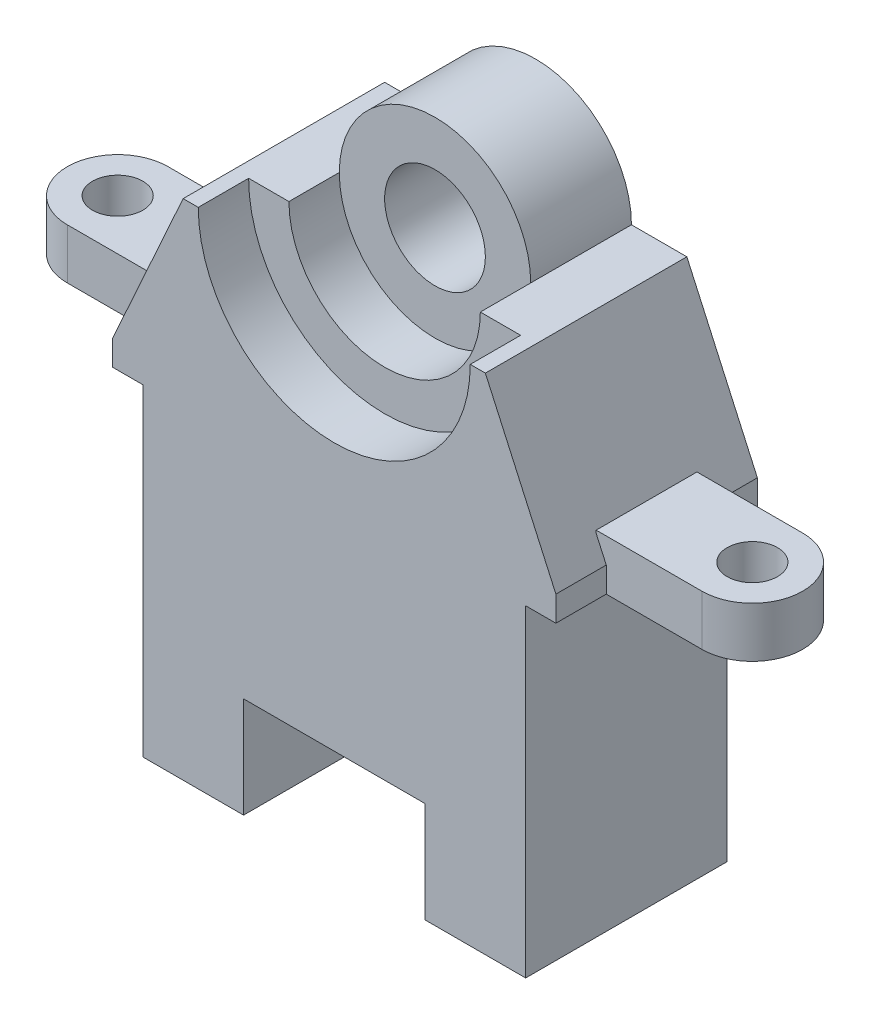
ISO-10303-21;
HEADER;
FILE_DESCRIPTION(('STEP AP214'),'2;1');
FILE_NAME('part.step','',(''),(''),'','','');
FILE_SCHEMA(('AUTOMOTIVE_DESIGN { 1 0 10303 214 1 1 1 1 }'));
ENDSEC;
DATA;
#1=APPLICATION_CONTEXT('core data for automotive mechanical design processes');
#2=APPLICATION_PROTOCOL_DEFINITION('international standard','automotive_design',2000,#1);
#3=PRODUCT_CONTEXT('',#1,'mechanical');
#4=PRODUCT('Part','Part','',(#3));
#5=PRODUCT_RELATED_PRODUCT_CATEGORY('part','',(#4));
#6=PRODUCT_DEFINITION_FORMATION('','',#4);
#7=PRODUCT_DEFINITION_CONTEXT('part definition',#1,'design');
#8=PRODUCT_DEFINITION('design','',#6,#7);
#9=PRODUCT_DEFINITION_SHAPE('','',#8);
#10=(LENGTH_UNIT() NAMED_UNIT(*) SI_UNIT(.MILLI.,.METRE.));
#11=(NAMED_UNIT(*) PLANE_ANGLE_UNIT() SI_UNIT($,.RADIAN.));
#12=(NAMED_UNIT(*) SI_UNIT($,.STERADIAN.) SOLID_ANGLE_UNIT());
#13=UNCERTAINTY_MEASURE_WITH_UNIT(LENGTH_MEASURE(1.E-05),#10,'distance_accuracy_value','');
#14=(GEOMETRIC_REPRESENTATION_CONTEXT(3) GLOBAL_UNCERTAINTY_ASSIGNED_CONTEXT((#13)) GLOBAL_UNIT_ASSIGNED_CONTEXT((#10,
#11,#12)) REPRESENTATION_CONTEXT('',''));
#15=CARTESIAN_POINT('',(0.,0.,0.));
#16=DIRECTION('',(0.,0.,1.));
#17=DIRECTION('',(1.,0.,0.));
#18=AXIS2_PLACEMENT_3D('',#15,#16,#17);
#19=CARTESIAN_POINT('',(38.,100.,0.));
#20=DIRECTION('',(0.,0.,1.));
#21=DIRECTION('',(1.,0.,0.));
#22=AXIS2_PLACEMENT_3D('',#19,#20,#21);
#23=CYLINDRICAL_SURFACE('',#22,19.);
#24=DIRECTION('',(0.,0.,1.));
#25=VECTOR('',#24,1.);
#26=CARTESIAN_POINT('',(19.,100.,0.));
#27=LINE('',#26,#25);
#28=CARTESIAN_POINT('',(19.,100.,0.));
#29=VERTEX_POINT('',#28);
#30=CARTESIAN_POINT('',(19.,100.,20.));
#31=VERTEX_POINT('',#30);
#32=EDGE_CURVE('E277',#29,#31,#27,.T.);
#33=ORIENTED_EDGE('',*,*,#32,.T.);
#34=CARTESIAN_POINT('',(38.,100.,20.));
#35=DIRECTION('',(0.,0.,1.));
#36=DIRECTION('',(1.,0.,0.));
#37=AXIS2_PLACEMENT_3D('',#34,#35,#36);
#38=CIRCLE('',#37,19.);
#39=CARTESIAN_POINT('',(57.,100.,20.));
#40=VERTEX_POINT('',#39);
#41=EDGE_CURVE('E1027',#40,#31,#38,.T.);
#42=ORIENTED_EDGE('',*,*,#41,.F.);
#43=DIRECTION('',(0.,0.,1.));
#44=VECTOR('',#43,1.);
#45=CARTESIAN_POINT('',(57.,100.,0.));
#46=LINE('',#45,#44);
#47=CARTESIAN_POINT('',(57.,100.,0.));
#48=VERTEX_POINT('',#47);
#49=EDGE_CURVE('E264',#48,#40,#46,.T.);
#50=ORIENTED_EDGE('',*,*,#49,.F.);
#51=CARTESIAN_POINT('',(38.,100.,0.));
#52=DIRECTION('',(0.,0.,1.));
#53=DIRECTION('',(1.,0.,0.));
#54=AXIS2_PLACEMENT_3D('',#51,#52,#53);
#55=CIRCLE('',#54,19.);
#56=EDGE_CURVE('E262',#48,#29,#55,.T.);
#57=ORIENTED_EDGE('',*,*,#56,.T.);
#58=EDGE_LOOP('',(#33,#42,#50,#57));
#59=FACE_BOUND('',#58,.T.);
#60=ADVANCED_FACE('F44',(#59),#23,.T.);
#61=CARTESIAN_POINT('',(38.,100.,0.));
#62=DIRECTION('',(0.,1.,0.));
#63=DIRECTION('',(0.,0.,1.));
#64=AXIS2_PLACEMENT_3D('',#61,#62,#63);
#65=PLANE('',#64);
#66=ORIENTED_EDGE('',*,*,#32,.F.);
#67=DIRECTION('',(-1.,0.,0.));
#68=VECTOR('',#67,1.);
#69=CARTESIAN_POINT('',(38.,100.,0.));
#70=LINE('',#69,#68);
#71=CARTESIAN_POINT('',(8.,100.,0.));
#72=VERTEX_POINT('',#71);
#73=EDGE_CURVE('E385',#29,#72,#70,.T.);
#74=ORIENTED_EDGE('',*,*,#73,.T.);
#75=DIRECTION('',(0.,0.,1.));
#76=VECTOR('',#75,1.);
#77=CARTESIAN_POINT('',(8.,100.,0.));
#78=LINE('',#77,#76);
#79=CARTESIAN_POINT('',(8.,100.,40.));
#80=VERTEX_POINT('',#79);
#81=EDGE_CURVE('E418',#72,#80,#78,.T.);
#82=ORIENTED_EDGE('',*,*,#81,.T.);
#83=DIRECTION('',(-1.,0.,0.));
#84=VECTOR('',#83,1.);
#85=CARTESIAN_POINT('',(38.,100.,40.));
#86=LINE('',#85,#84);
#87=CARTESIAN_POINT('',(11.,100.,40.));
#88=VERTEX_POINT('',#87);
#89=EDGE_CURVE('E397',#88,#80,#86,.T.);
#90=ORIENTED_EDGE('',*,*,#89,.F.);
#91=DIRECTION('',(0.,0.,1.));
#92=VECTOR('',#91,1.);
#93=CARTESIAN_POINT('',(11.,100.,30.));
#94=LINE('',#93,#92);
#95=CARTESIAN_POINT('',(11.,100.,30.));
#96=VERTEX_POINT('',#95);
#97=EDGE_CURVE('E272',#96,#88,#94,.T.);
#98=ORIENTED_EDGE('',*,*,#97,.F.);
#99=DIRECTION('',(-1.,0.,0.));
#100=VECTOR('',#99,1.);
#101=CARTESIAN_POINT('',(11.,100.,30.));
#102=LINE('',#101,#100);
#103=CARTESIAN_POINT('',(19.,100.,30.));
#104=VERTEX_POINT('',#103);
#105=EDGE_CURVE('E268',#104,#96,#102,.T.);
#106=ORIENTED_EDGE('',*,*,#105,.F.);
#107=EDGE_CURVE('E254',#31,#104,#27,.T.);
#108=ORIENTED_EDGE('',*,*,#107,.F.);
#109=EDGE_LOOP('',(#66,#74,#82,#90,#98,#106,#108));
#110=FACE_BOUND('',#109,.T.);
#111=ADVANCED_FACE('F531',(#110),#65,.T.);
#112=CARTESIAN_POINT('',(82.,64.,0.));
#113=DIRECTION('',(1.,0.,0.));
#114=DIRECTION('',(0.,0.,-1.));
#115=AXIS2_PLACEMENT_3D('',#112,#113,#114);
#116=PLANE('',#115);
#117=DIRECTION('',(0.,-1.,0.));
#118=VECTOR('',#117,1.);
#119=CARTESIAN_POINT('',(82.,69.,30.));
#120=LINE('',#119,#118);
#121=CARTESIAN_POINT('',(82.,69.,30.));
#122=VERTEX_POINT('',#121);
#123=CARTESIAN_POINT('',(82.,64.,30.));
#124=VERTEX_POINT('',#123);
#125=EDGE_CURVE('E315',#122,#124,#120,.T.);
#126=ORIENTED_EDGE('',*,*,#125,.F.);
#127=DIRECTION('',(0.,0.,1.));
#128=VECTOR('',#127,1.);
#129=CARTESIAN_POINT('',(82.,69.,0.));
#130=LINE('',#129,#128);
#131=CARTESIAN_POINT('',(82.,69.,40.));
#132=VERTEX_POINT('',#131);
#133=EDGE_CURVE('E426',#122,#132,#130,.T.);
#134=ORIENTED_EDGE('',*,*,#133,.T.);
#135=DIRECTION('',(0.,1.,0.));
#136=VECTOR('',#135,1.);
#137=CARTESIAN_POINT('',(82.,64.,40.));
#138=LINE('',#137,#136);
#139=CARTESIAN_POINT('',(82.,64.,40.));
#140=VERTEX_POINT('',#139);
#141=EDGE_CURVE('E371',#140,#132,#138,.T.);
#142=ORIENTED_EDGE('',*,*,#141,.F.);
#143=DIRECTION('',(0.,0.,1.));
#144=VECTOR('',#143,1.);
#145=CARTESIAN_POINT('',(82.,64.,0.));
#146=LINE('',#145,#144);
#147=EDGE_CURVE('E393',#124,#140,#146,.T.);
#148=ORIENTED_EDGE('',*,*,#147,.F.);
#149=EDGE_LOOP('',(#126,#134,#142,#148));
#150=FACE_BOUND('',#149,.T.);
#151=ADVANCED_FACE('F540',(#150),#116,.T.);
#152=CARTESIAN_POINT('',(-6.,64.,0.));
#153=DIRECTION('',(-1.,0.,0.));
#154=DIRECTION('',(0.,0.,1.));
#155=AXIS2_PLACEMENT_3D('',#152,#153,#154);
#156=PLANE('',#155);
#157=DIRECTION('',(0.,-1.,0.));
#158=VECTOR('',#157,1.);
#159=CARTESIAN_POINT('',(-6.,69.,10.));
#160=LINE('',#159,#158);
#161=CARTESIAN_POINT('',(-6.,69.,10.));
#162=VERTEX_POINT('',#161);
#163=CARTESIAN_POINT('',(-6.,64.,10.));
#164=VERTEX_POINT('',#163);
#165=EDGE_CURVE('E356',#162,#164,#160,.T.);
#166=ORIENTED_EDGE('',*,*,#165,.F.);
#167=DIRECTION('',(0.,0.,1.));
#168=VECTOR('',#167,1.);
#169=CARTESIAN_POINT('',(-6.,69.,0.));
#170=LINE('',#169,#168);
#171=CARTESIAN_POINT('',(-6.,69.,0.));
#172=VERTEX_POINT('',#171);
#173=EDGE_CURVE('E412',#172,#162,#170,.T.);
#174=ORIENTED_EDGE('',*,*,#173,.F.);
#175=DIRECTION('',(0.,-1.,0.));
#176=VECTOR('',#175,1.);
#177=CARTESIAN_POINT('',(-6.,64.,0.));
#178=LINE('',#177,#176);
#179=CARTESIAN_POINT('',(-6.,64.,0.));
#180=VERTEX_POINT('',#179);
#181=EDGE_CURVE('E389',#172,#180,#178,.T.);
#182=ORIENTED_EDGE('',*,*,#181,.T.);
#183=DIRECTION('',(0.,0.,1.));
#184=VECTOR('',#183,1.);
#185=CARTESIAN_POINT('',(-6.,64.,0.));
#186=LINE('',#185,#184);
#187=EDGE_CURVE('E413',#180,#164,#186,.T.);
#188=ORIENTED_EDGE('',*,*,#187,.T.);
#189=EDGE_LOOP('',(#166,#174,#182,#188));
#190=FACE_BOUND('',#189,.T.);
#191=ADVANCED_FACE('F499',(#190),#156,.T.);
#192=CARTESIAN_POINT('',(20.,0.,40.));
#193=DIRECTION('',(0.,1.,0.));
#194=DIRECTION('',(0.,0.,1.));
#195=AXIS2_PLACEMENT_3D('',#192,#193,#194);
#196=PLANE('',#195);
#197=DIRECTION('',(1.,0.,0.));
#198=VECTOR('',#197,1.);
#199=CARTESIAN_POINT('',(20.,0.,0.));
#200=LINE('',#199,#198);
#201=CARTESIAN_POINT('',(0.,0.,0.));
#202=VERTEX_POINT('',#201);
#203=CARTESIAN_POINT('',(20.,0.,0.));
#204=VERTEX_POINT('',#203);
#205=EDGE_CURVE('E411',#202,#204,#200,.T.);
#206=ORIENTED_EDGE('',*,*,#205,.T.);
#207=DIRECTION('',(0.,0.,-1.));
#208=VECTOR('',#207,1.);
#209=CARTESIAN_POINT('',(20.,0.,40.));
#210=LINE('',#209,#208);
#211=CARTESIAN_POINT('',(20.,0.,40.));
#212=VERTEX_POINT('',#211);
#213=EDGE_CURVE('E481',#212,#204,#210,.T.);
#214=ORIENTED_EDGE('',*,*,#213,.F.);
#215=DIRECTION('',(1.,0.,0.));
#216=VECTOR('',#215,1.);
#217=CARTESIAN_POINT('',(20.,0.,40.));
#218=LINE('',#217,#216);
#219=CARTESIAN_POINT('',(0.,0.,40.));
#220=VERTEX_POINT('',#219);
#221=EDGE_CURVE('E435',#220,#212,#218,.T.);
#222=ORIENTED_EDGE('',*,*,#221,.F.);
#223=DIRECTION('',(0.,0.,-1.));
#224=VECTOR('',#223,1.);
#225=CARTESIAN_POINT('',(0.,0.,40.));
#226=LINE('',#225,#224);
#227=EDGE_CURVE('E449',#220,#202,#226,.T.);
#228=ORIENTED_EDGE('',*,*,#227,.T.);
#229=EDGE_LOOP('',(#206,#214,#222,#228));
#230=FACE_BOUND('',#229,.T.);
#231=ADVANCED_FACE('F50',(#230),#196,.F.);
#232=CARTESIAN_POINT('',(20.,20.,40.));
#233=DIRECTION('',(-1.,0.,0.));
#234=DIRECTION('',(0.,0.,1.));
#235=AXIS2_PLACEMENT_3D('',#232,#233,#234);
#236=PLANE('',#235);
#237=DIRECTION('',(0.,1.,0.));
#238=VECTOR('',#237,1.);
#239=CARTESIAN_POINT('',(20.,20.,0.));
#240=LINE('',#239,#238);
#241=CARTESIAN_POINT('',(20.,20.,0.));
#242=VERTEX_POINT('',#241);
#243=EDGE_CURVE('E451',#204,#242,#240,.T.);
#244=ORIENTED_EDGE('',*,*,#243,.T.);
#245=DIRECTION('',(0.,0.,-1.));
#246=VECTOR('',#245,1.);
#247=CARTESIAN_POINT('',(20.,20.,40.));
#248=LINE('',#247,#246);
#249=CARTESIAN_POINT('',(20.,20.,40.));
#250=VERTEX_POINT('',#249);
#251=EDGE_CURVE('E476',#250,#242,#248,.T.);
#252=ORIENTED_EDGE('',*,*,#251,.F.);
#253=DIRECTION('',(0.,1.,0.));
#254=VECTOR('',#253,1.);
#255=CARTESIAN_POINT('',(20.,20.,40.));
#256=LINE('',#255,#254);
#257=EDGE_CURVE('E434',#212,#250,#256,.T.);
#258=ORIENTED_EDGE('',*,*,#257,.F.);
#259=ORIENTED_EDGE('',*,*,#213,.T.);
#260=EDGE_LOOP('',(#244,#252,#258,#259));
#261=FACE_BOUND('',#260,.T.);
#262=ADVANCED_FACE('F892',(#261),#236,.F.);
#263=CARTESIAN_POINT('',(56.,20.,40.));
#264=DIRECTION('',(0.,1.,0.));
#265=DIRECTION('',(0.,0.,1.));
#266=AXIS2_PLACEMENT_3D('',#263,#264,#265);
#267=PLANE('',#266);
#268=DIRECTION('',(1.,0.,0.));
#269=VECTOR('',#268,1.);
#270=CARTESIAN_POINT('',(56.,20.,0.));
#271=LINE('',#270,#269);
#272=CARTESIAN_POINT('',(56.,20.,0.));
#273=VERTEX_POINT('',#272);
#274=EDGE_CURVE('E454',#242,#273,#271,.T.);
#275=ORIENTED_EDGE('',*,*,#274,.T.);
#276=DIRECTION('',(0.,0.,-1.));
#277=VECTOR('',#276,1.);
#278=CARTESIAN_POINT('',(56.,20.,40.));
#279=LINE('',#278,#277);
#280=CARTESIAN_POINT('',(56.,20.,40.));
#281=VERTEX_POINT('',#280);
#282=EDGE_CURVE('E475',#281,#273,#279,.T.);
#283=ORIENTED_EDGE('',*,*,#282,.F.);
#284=DIRECTION('',(1.,0.,0.));
#285=VECTOR('',#284,1.);
#286=CARTESIAN_POINT('',(56.,20.,40.));
#287=LINE('',#286,#285);
#288=EDGE_CURVE('E438',#250,#281,#287,.T.);
#289=ORIENTED_EDGE('',*,*,#288,.F.);
#290=ORIENTED_EDGE('',*,*,#251,.T.);
#291=EDGE_LOOP('',(#275,#283,#289,#290));
#292=FACE_BOUND('',#291,.T.);
#293=ADVANCED_FACE('F885',(#292),#267,.F.);
#294=CARTESIAN_POINT('',(56.,0.,40.));
#295=DIRECTION('',(1.,0.,0.));
#296=DIRECTION('',(0.,0.,-1.));
#297=AXIS2_PLACEMENT_3D('',#294,#295,#296);
#298=PLANE('',#297);
#299=DIRECTION('',(0.,-1.,0.));
#300=VECTOR('',#299,1.);
#301=CARTESIAN_POINT('',(56.,0.,0.));
#302=LINE('',#301,#300);
#303=CARTESIAN_POINT('',(56.,0.,0.));
#304=VERTEX_POINT('',#303);
#305=EDGE_CURVE('E455',#273,#304,#302,.T.);
#306=ORIENTED_EDGE('',*,*,#305,.T.);
#307=DIRECTION('',(0.,0.,-1.));
#308=VECTOR('',#307,1.);
#309=CARTESIAN_POINT('',(56.,0.,40.));
#310=LINE('',#309,#308);
#311=CARTESIAN_POINT('',(56.,0.,40.));
#312=VERTEX_POINT('',#311);
#313=EDGE_CURVE('E472',#312,#304,#310,.T.);
#314=ORIENTED_EDGE('',*,*,#313,.F.);
#315=DIRECTION('',(0.,-1.,0.));
#316=VECTOR('',#315,1.);
#317=CARTESIAN_POINT('',(56.,0.,40.));
#318=LINE('',#317,#316);
#319=EDGE_CURVE('E439',#281,#312,#318,.T.);
#320=ORIENTED_EDGE('',*,*,#319,.F.);
#321=ORIENTED_EDGE('',*,*,#282,.T.);
#322=EDGE_LOOP('',(#306,#314,#320,#321));
#323=FACE_BOUND('',#322,.T.);
#324=ADVANCED_FACE('F871',(#323),#298,.F.);
#325=CARTESIAN_POINT('',(76.,0.,40.));
#326=DIRECTION('',(0.,1.,0.));
#327=DIRECTION('',(0.,0.,1.));
#328=AXIS2_PLACEMENT_3D('',#325,#326,#327);
#329=PLANE('',#328);
#330=DIRECTION('',(1.,0.,0.));
#331=VECTOR('',#330,1.);
#332=CARTESIAN_POINT('',(76.,0.,0.));
#333=LINE('',#332,#331);
#334=CARTESIAN_POINT('',(76.,0.,0.));
#335=VERTEX_POINT('',#334);
#336=EDGE_CURVE('E460',#304,#335,#333,.T.);
#337=ORIENTED_EDGE('',*,*,#336,.T.);
#338=DIRECTION('',(0.,0.,-1.));
#339=VECTOR('',#338,1.);
#340=CARTESIAN_POINT('',(76.,0.,40.));
#341=LINE('',#340,#339);
#342=CARTESIAN_POINT('',(76.,0.,40.));
#343=VERTEX_POINT('',#342);
#344=EDGE_CURVE('E469',#343,#335,#341,.T.);
#345=ORIENTED_EDGE('',*,*,#344,.F.);
#346=DIRECTION('',(1.,0.,0.));
#347=VECTOR('',#346,1.);
#348=CARTESIAN_POINT('',(76.,0.,40.));
#349=LINE('',#348,#347);
#350=EDGE_CURVE('E445',#312,#343,#349,.T.);
#351=ORIENTED_EDGE('',*,*,#350,.F.);
#352=ORIENTED_EDGE('',*,*,#313,.T.);
#353=EDGE_LOOP('',(#337,#345,#351,#352));
#354=FACE_BOUND('',#353,.T.);
#355=ADVANCED_FACE('F858',(#354),#329,.F.);
#356=CARTESIAN_POINT('',(76.,64.,40.));
#357=DIRECTION('',(-1.,0.,0.));
#358=DIRECTION('',(0.,0.,1.));
#359=AXIS2_PLACEMENT_3D('',#356,#357,#358);
#360=PLANE('',#359);
#361=DIRECTION('',(0.,1.,0.));
#362=VECTOR('',#361,1.);
#363=CARTESIAN_POINT('',(76.,64.,0.));
#364=LINE('',#363,#362);
#365=CARTESIAN_POINT('',(76.,64.,0.));
#366=VERTEX_POINT('',#365);
#367=EDGE_CURVE('E459',#335,#366,#364,.T.);
#368=ORIENTED_EDGE('',*,*,#367,.T.);
#369=DIRECTION('',(0.,0.,-1.));
#370=VECTOR('',#369,1.);
#371=CARTESIAN_POINT('',(76.,64.,40.));
#372=LINE('',#371,#370);
#373=CARTESIAN_POINT('',(76.,64.,40.));
#374=VERTEX_POINT('',#373);
#375=EDGE_CURVE('E467',#374,#366,#372,.T.);
#376=ORIENTED_EDGE('',*,*,#375,.F.);
#377=DIRECTION('',(0.,1.,0.));
#378=VECTOR('',#377,1.);
#379=CARTESIAN_POINT('',(76.,64.,40.));
#380=LINE('',#379,#378);
#381=EDGE_CURVE('E443',#343,#374,#380,.T.);
#382=ORIENTED_EDGE('',*,*,#381,.F.);
#383=ORIENTED_EDGE('',*,*,#344,.T.);
#384=EDGE_LOOP('',(#368,#376,#382,#383));
#385=FACE_BOUND('',#384,.T.);
#386=ADVANCED_FACE('F849',(#385),#360,.F.);
#387=CARTESIAN_POINT('',(0.,0.,40.));
#388=DIRECTION('',(1.,0.,0.));
#389=DIRECTION('',(0.,0.,-1.));
#390=AXIS2_PLACEMENT_3D('',#387,#388,#389);
#391=PLANE('',#390);
#392=DIRECTION('',(0.,-1.,0.));
#393=VECTOR('',#392,1.);
#394=CARTESIAN_POINT('',(0.,0.,0.));
#395=LINE('',#394,#393);
#396=CARTESIAN_POINT('',(0.,64.,0.));
#397=VERTEX_POINT('',#396);
#398=EDGE_CURVE('E436',#397,#202,#395,.T.);
#399=ORIENTED_EDGE('',*,*,#398,.T.);
#400=ORIENTED_EDGE('',*,*,#227,.F.);
#401=DIRECTION('',(0.,-1.,0.));
#402=VECTOR('',#401,1.);
#403=CARTESIAN_POINT('',(0.,0.,40.));
#404=LINE('',#403,#402);
#405=CARTESIAN_POINT('',(0.,64.,40.));
#406=VERTEX_POINT('',#405);
#407=EDGE_CURVE('E447',#406,#220,#404,.T.);
#408=ORIENTED_EDGE('',*,*,#407,.F.);
#409=DIRECTION('',(0.,0.,-1.));
#410=VECTOR('',#409,1.);
#411=CARTESIAN_POINT('',(0.,64.,40.));
#412=LINE('',#411,#410);
#413=EDGE_CURVE('E463',#406,#397,#412,.T.);
#414=ORIENTED_EDGE('',*,*,#413,.T.);
#415=EDGE_LOOP('',(#399,#400,#408,#414));
#416=FACE_BOUND('',#415,.T.);
#417=ADVANCED_FACE('F703',(#416),#391,.F.);
#418=CARTESIAN_POINT('',(0.,0.,40.));
#419=DIRECTION('',(0.,0.,-1.));
#420=DIRECTION('',(-1.,0.,0.));
#421=AXIS2_PLACEMENT_3D('',#418,#419,#420);
#422=PLANE('',#421);
#423=CARTESIAN_POINT('',(68.,100.,40.));
#424=VERTEX_POINT('',#423);
#425=CARTESIAN_POINT('',(65.,100.,40.));
#426=VERTEX_POINT('',#425);
#427=EDGE_CURVE('E399',#424,#426,#86,.T.);
#428=ORIENTED_EDGE('',*,*,#427,.T.);
#429=CARTESIAN_POINT('',(38.,100.,40.));
#430=DIRECTION('',(0.,0.,1.));
#431=DIRECTION('',(1.,0.,0.));
#432=AXIS2_PLACEMENT_3D('',#429,#430,#431);
#433=CIRCLE('',#432,27.);
#434=EDGE_CURVE('E273',#88,#426,#433,.T.);
#435=ORIENTED_EDGE('',*,*,#434,.F.);
#436=ORIENTED_EDGE('',*,*,#89,.T.);
#437=DIRECTION('',(-0.411586722426498,-0.911370599658675,0.));
#438=VECTOR('',#437,1.);
#439=CARTESIAN_POINT('',(8.,100.,40.));
#440=LINE('',#439,#438);
#441=CARTESIAN_POINT('',(-6.,69.,40.));
#442=VERTEX_POINT('',#441);
#443=EDGE_CURVE('E402',#80,#442,#440,.T.);
#444=ORIENTED_EDGE('',*,*,#443,.T.);
#445=DIRECTION('',(0.,-1.,0.));
#446=VECTOR('',#445,1.);
#447=CARTESIAN_POINT('',(-6.,64.,40.));
#448=LINE('',#447,#446);
#449=CARTESIAN_POINT('',(-6.,64.,40.));
#450=VERTEX_POINT('',#449);
#451=EDGE_CURVE('E404',#442,#450,#448,.T.);
#452=ORIENTED_EDGE('',*,*,#451,.T.);
#453=DIRECTION('',(1.,0.,0.));
#454=VECTOR('',#453,1.);
#455=CARTESIAN_POINT('',(0.,64.,40.));
#456=LINE('',#455,#454);
#457=EDGE_CURVE('E409',#450,#406,#456,.T.);
#458=ORIENTED_EDGE('',*,*,#457,.T.);
#459=ORIENTED_EDGE('',*,*,#407,.T.);
#460=ORIENTED_EDGE('',*,*,#221,.T.);
#461=ORIENTED_EDGE('',*,*,#257,.T.);
#462=ORIENTED_EDGE('',*,*,#288,.T.);
#463=ORIENTED_EDGE('',*,*,#319,.T.);
#464=ORIENTED_EDGE('',*,*,#350,.T.);
#465=ORIENTED_EDGE('',*,*,#381,.T.);
#466=EDGE_CURVE('E407',#374,#140,#456,.T.);
#467=ORIENTED_EDGE('',*,*,#466,.T.);
#468=ORIENTED_EDGE('',*,*,#141,.T.);
#469=DIRECTION('',(-0.411586722426498,0.911370599658675,0.));
#470=VECTOR('',#469,1.);
#471=CARTESIAN_POINT('',(82.,69.,40.));
#472=LINE('',#471,#470);
#473=EDGE_CURVE('E394',#132,#424,#472,.T.);
#474=ORIENTED_EDGE('',*,*,#473,.T.);
#475=EDGE_LOOP('',(#428,#435,#436,#444,#452,#458,#459,#460,#461,#462,#463,#464,#465,#467,#468,#474));
#476=FACE_BOUND('',#475,.T.);
#477=ADVANCED_FACE('F652',(#476),#422,.F.);
#478=CARTESIAN_POINT('',(0.,0.,0.));
#479=DIRECTION('',(0.,0.,-1.));
#480=DIRECTION('',(-1.,0.,0.));
#481=AXIS2_PLACEMENT_3D('',#478,#479,#480);
#482=PLANE('',#481);
#483=CARTESIAN_POINT('',(38.,100.,0.));
#484=DIRECTION('',(0.,0.,1.));
#485=DIRECTION('',(1.,0.,0.));
#486=AXIS2_PLACEMENT_3D('',#483,#484,#485);
#487=CIRCLE('',#486,10.);
#488=CARTESIAN_POINT('',(48.,100.,0.));
#489=VERTEX_POINT('',#488);
#490=EDGE_CURVE('E253',#489,#489,#487,.T.);
#491=ORIENTED_EDGE('',*,*,#490,.T.);
#492=EDGE_LOOP('',(#491));
#493=FACE_BOUND('',#492,.T.);
#494=ORIENTED_EDGE('',*,*,#73,.F.);
#495=ORIENTED_EDGE('',*,*,#56,.F.);
#496=CARTESIAN_POINT('',(68.,100.,0.));
#497=VERTEX_POINT('',#496);
#498=EDGE_CURVE('E384',#497,#48,#70,.T.);
#499=ORIENTED_EDGE('',*,*,#498,.F.);
#500=DIRECTION('',(-0.411586722426498,0.911370599658675,0.));
#501=VECTOR('',#500,1.);
#502=CARTESIAN_POINT('',(82.,69.,0.));
#503=LINE('',#502,#501);
#504=CARTESIAN_POINT('',(82.,69.,0.));
#505=VERTEX_POINT('',#504);
#506=EDGE_CURVE('E378',#505,#497,#503,.T.);
#507=ORIENTED_EDGE('',*,*,#506,.F.);
#508=DIRECTION('',(0.,1.,0.));
#509=VECTOR('',#508,1.);
#510=CARTESIAN_POINT('',(82.,64.,0.));
#511=LINE('',#510,#509);
#512=CARTESIAN_POINT('',(82.,64.,0.));
#513=VERTEX_POINT('',#512);
#514=EDGE_CURVE('E374',#513,#505,#511,.T.);
#515=ORIENTED_EDGE('',*,*,#514,.F.);
#516=DIRECTION('',(1.,0.,0.));
#517=VECTOR('',#516,1.);
#518=CARTESIAN_POINT('',(0.,64.,0.));
#519=LINE('',#518,#517);
#520=EDGE_CURVE('E376',#366,#513,#519,.T.);
#521=ORIENTED_EDGE('',*,*,#520,.F.);
#522=ORIENTED_EDGE('',*,*,#367,.F.);
#523=ORIENTED_EDGE('',*,*,#336,.F.);
#524=ORIENTED_EDGE('',*,*,#305,.F.);
#525=ORIENTED_EDGE('',*,*,#274,.F.);
#526=ORIENTED_EDGE('',*,*,#243,.F.);
#527=ORIENTED_EDGE('',*,*,#205,.F.);
#528=ORIENTED_EDGE('',*,*,#398,.F.);
#529=EDGE_CURVE('E375',#180,#397,#519,.T.);
#530=ORIENTED_EDGE('',*,*,#529,.F.);
#531=ORIENTED_EDGE('',*,*,#181,.F.);
#532=DIRECTION('',(-0.411586722426498,-0.911370599658675,0.));
#533=VECTOR('',#532,1.);
#534=CARTESIAN_POINT('',(8.,100.,0.));
#535=LINE('',#534,#533);
#536=EDGE_CURVE('E383',#72,#172,#535,.T.);
#537=ORIENTED_EDGE('',*,*,#536,.F.);
#538=EDGE_LOOP('',(#494,#495,#499,#507,#515,#521,#522,#523,#524,#525,#526,#527,#528,#530,#531,#537));
#539=FACE_BOUND('',#538,.T.);
#540=ADVANCED_FACE('F503',(#493,#539),#482,.T.);
#541=CARTESIAN_POINT('',(0.,64.,0.));
#542=DIRECTION('',(0.,-1.,0.));
#543=DIRECTION('',(0.,0.,-1.));
#544=AXIS2_PLACEMENT_3D('',#541,#542,#543);
#545=PLANE('',#544);
#546=CARTESIAN_POINT('',(-25.,64.,20.));
#547=DIRECTION('',(0.,1.,0.));
#548=DIRECTION('',(0.,0.,1.));
#549=AXIS2_PLACEMENT_3D('',#546,#547,#548);
#550=CIRCLE('',#549,5.);
#551=CARTESIAN_POINT('',(-25.,64.,25.));
#552=VERTEX_POINT('',#551);
#553=EDGE_CURVE('E328',#552,#552,#550,.T.);
#554=ORIENTED_EDGE('',*,*,#553,.T.);
#555=EDGE_LOOP('',(#554));
#556=FACE_BOUND('',#555,.T.);
#557=ORIENTED_EDGE('',*,*,#413,.F.);
#558=ORIENTED_EDGE('',*,*,#457,.F.);
#559=CARTESIAN_POINT('',(-6.,64.,30.));
#560=VERTEX_POINT('',#559);
#561=EDGE_CURVE('E414',#560,#450,#186,.T.);
#562=ORIENTED_EDGE('',*,*,#561,.F.);
#563=DIRECTION('',(1.,0.,0.));
#564=VECTOR('',#563,1.);
#565=CARTESIAN_POINT('',(-25.,64.,30.));
#566=LINE('',#565,#564);
#567=CARTESIAN_POINT('',(-25.,64.,30.));
#568=VERTEX_POINT('',#567);
#569=EDGE_CURVE('E368',#568,#560,#566,.T.);
#570=ORIENTED_EDGE('',*,*,#569,.F.);
#571=CARTESIAN_POINT('',(-25.,64.,20.));
#572=DIRECTION('',(0.,1.,0.));
#573=DIRECTION('',(0.,0.,1.));
#574=AXIS2_PLACEMENT_3D('',#571,#572,#573);
#575=CIRCLE('',#574,10.);
#576=CARTESIAN_POINT('',(-25.,64.,10.));
#577=VERTEX_POINT('',#576);
#578=EDGE_CURVE('E332',#577,#568,#575,.T.);
#579=ORIENTED_EDGE('',*,*,#578,.F.);
#580=DIRECTION('',(1.,0.,0.));
#581=VECTOR('',#580,1.);
#582=CARTESIAN_POINT('',(-25.,64.,10.));
#583=LINE('',#582,#581);
#584=EDGE_CURVE('E363',#577,#164,#583,.T.);
#585=ORIENTED_EDGE('',*,*,#584,.T.);
#586=ORIENTED_EDGE('',*,*,#187,.F.);
#587=ORIENTED_EDGE('',*,*,#529,.T.);
#588=EDGE_LOOP('',(#557,#558,#562,#570,#579,#585,#586,#587));
#589=FACE_BOUND('',#588,.T.);
#590=ADVANCED_FACE('F508',(#556,#589),#545,.T.);
#591=CARTESIAN_POINT('',(101.,64.,20.));
#592=DIRECTION('',(0.,1.,0.));
#593=DIRECTION('',(0.,0.,1.));
#594=AXIS2_PLACEMENT_3D('',#591,#592,#593);
#595=CIRCLE('',#594,5.);
#596=CARTESIAN_POINT('',(101.,64.,25.));
#597=VERTEX_POINT('',#596);
#598=EDGE_CURVE('E280',#597,#597,#595,.T.);
#599=ORIENTED_EDGE('',*,*,#598,.T.);
#600=EDGE_LOOP('',(#599));
#601=FACE_BOUND('',#600,.T.);
#602=ORIENTED_EDGE('',*,*,#466,.F.);
#603=ORIENTED_EDGE('',*,*,#375,.T.);
#604=ORIENTED_EDGE('',*,*,#520,.T.);
#605=CARTESIAN_POINT('',(82.,64.,10.));
#606=VERTEX_POINT('',#605);
#607=EDGE_CURVE('E429',#513,#606,#146,.T.);
#608=ORIENTED_EDGE('',*,*,#607,.T.);
#609=DIRECTION('',(-1.,0.,0.));
#610=VECTOR('',#609,1.);
#611=CARTESIAN_POINT('',(101.,64.,10.));
#612=LINE('',#611,#610);
#613=CARTESIAN_POINT('',(101.,64.,10.));
#614=VERTEX_POINT('',#613);
#615=EDGE_CURVE('E322',#614,#606,#612,.T.);
#616=ORIENTED_EDGE('',*,*,#615,.F.);
#617=CARTESIAN_POINT('',(101.,64.,20.));
#618=DIRECTION('',(0.,1.,0.));
#619=DIRECTION('',(0.,0.,1.));
#620=AXIS2_PLACEMENT_3D('',#617,#618,#619);
#621=CIRCLE('',#620,10.);
#622=CARTESIAN_POINT('',(101.,64.,30.));
#623=VERTEX_POINT('',#622);
#624=EDGE_CURVE('E286',#623,#614,#621,.T.);
#625=ORIENTED_EDGE('',*,*,#624,.F.);
#626=DIRECTION('',(-1.,0.,0.));
#627=VECTOR('',#626,1.);
#628=CARTESIAN_POINT('',(101.,64.,30.));
#629=LINE('',#628,#627);
#630=EDGE_CURVE('E314',#623,#124,#629,.T.);
#631=ORIENTED_EDGE('',*,*,#630,.T.);
#632=ORIENTED_EDGE('',*,*,#147,.T.);
#633=EDGE_LOOP('',(#602,#603,#604,#608,#616,#625,#631,#632));
#634=FACE_BOUND('',#633,.T.);
#635=ADVANCED_FACE('F724',(#601,#634),#545,.T.);
#636=DIRECTION('',(0.,1.,0.));
#637=VECTOR('',#636,1.);
#638=CARTESIAN_POINT('',(-6.,64.,30.));
#639=LINE('',#638,#637);
#640=CARTESIAN_POINT('',(-6.,69.,30.));
#641=VERTEX_POINT('',#640);
#642=EDGE_CURVE('E354',#560,#641,#639,.T.);
#643=ORIENTED_EDGE('',*,*,#642,.F.);
#644=ORIENTED_EDGE('',*,*,#561,.T.);
#645=ORIENTED_EDGE('',*,*,#451,.F.);
#646=EDGE_CURVE('E419',#641,#442,#170,.T.);
#647=ORIENTED_EDGE('',*,*,#646,.F.);
#648=EDGE_LOOP('',(#643,#644,#645,#647));
#649=FACE_BOUND('',#648,.T.);
#650=ADVANCED_FACE('F725',(#649),#156,.T.);
#651=CARTESIAN_POINT('',(8.,100.,0.));
#652=DIRECTION('',(-0.911370599658675,0.411586722426498,0.));
#653=DIRECTION('',(-0.411586722426498,-0.911370599658675,0.));
#654=AXIS2_PLACEMENT_3D('',#651,#652,#653);
#655=PLANE('',#654);
#656=DIRECTION('',(-0.411586722426498,-0.911370599658675,0.));
#657=VECTOR('',#656,1.);
#658=CARTESIAN_POINT('',(8.,100.,10.));
#659=LINE('',#658,#657);
#660=CARTESIAN_POINT('',(-4.,73.4285714285714,10.));
#661=VERTEX_POINT('',#660);
#662=EDGE_CURVE('E351',#661,#162,#659,.T.);
#663=ORIENTED_EDGE('',*,*,#662,.F.);
#664=DIRECTION('',(0.,0.,-1.));
#665=VECTOR('',#664,1.);
#666=CARTESIAN_POINT('',(-4.,73.4285714285714,0.));
#667=LINE('',#666,#665);
#668=CARTESIAN_POINT('',(-4.,73.4285714285714,30.));
#669=VERTEX_POINT('',#668);
#670=EDGE_CURVE('E52',#669,#661,#667,.T.);
#671=ORIENTED_EDGE('',*,*,#670,.F.);
#672=DIRECTION('',(0.411586722426498,0.911370599658675,0.));
#673=VECTOR('',#672,1.);
#674=CARTESIAN_POINT('',(8.,100.,30.));
#675=LINE('',#674,#673);
#676=EDGE_CURVE('E346',#641,#669,#675,.T.);
#677=ORIENTED_EDGE('',*,*,#676,.F.);
#678=ORIENTED_EDGE('',*,*,#646,.T.);
#679=ORIENTED_EDGE('',*,*,#443,.F.);
#680=ORIENTED_EDGE('',*,*,#81,.F.);
#681=ORIENTED_EDGE('',*,*,#536,.T.);
#682=ORIENTED_EDGE('',*,*,#173,.T.);
#683=EDGE_LOOP('',(#663,#671,#677,#678,#679,#680,#681,#682));
#684=FACE_BOUND('',#683,.T.);
#685=ADVANCED_FACE('F492',(#684),#655,.T.);
#686=ORIENTED_EDGE('',*,*,#49,.T.);
#687=CARTESIAN_POINT('',(57.,100.,30.));
#688=VERTEX_POINT('',#687);
#689=EDGE_CURVE('E249',#40,#688,#46,.T.);
#690=ORIENTED_EDGE('',*,*,#689,.T.);
#691=CARTESIAN_POINT('',(65.,100.,30.));
#692=VERTEX_POINT('',#691);
#693=EDGE_CURVE('E265',#692,#688,#102,.T.);
#694=ORIENTED_EDGE('',*,*,#693,.F.);
#695=DIRECTION('',(0.,0.,1.));
#696=VECTOR('',#695,1.);
#697=CARTESIAN_POINT('',(65.,100.,30.));
#698=LINE('',#697,#696);
#699=EDGE_CURVE('E269',#692,#426,#698,.T.);
#700=ORIENTED_EDGE('',*,*,#699,.T.);
#701=ORIENTED_EDGE('',*,*,#427,.F.);
#702=DIRECTION('',(0.,0.,1.));
#703=VECTOR('',#702,1.);
#704=CARTESIAN_POINT('',(68.,100.,0.));
#705=LINE('',#704,#703);
#706=EDGE_CURVE('E422',#497,#424,#705,.T.);
#707=ORIENTED_EDGE('',*,*,#706,.F.);
#708=ORIENTED_EDGE('',*,*,#498,.T.);
#709=EDGE_LOOP('',(#686,#690,#694,#700,#701,#707,#708));
#710=FACE_BOUND('',#709,.T.);
#711=ADVANCED_FACE('F260',(#710),#65,.T.);
#712=CARTESIAN_POINT('',(82.,69.,0.));
#713=DIRECTION('',(0.911370599658675,0.411586722426498,0.));
#714=DIRECTION('',(-0.411586722426498,0.911370599658675,0.));
#715=AXIS2_PLACEMENT_3D('',#712,#713,#714);
#716=PLANE('',#715);
#717=DIRECTION('',(0.411586722426498,-0.911370599658675,0.));
#718=VECTOR('',#717,1.);
#719=CARTESIAN_POINT('',(82.,69.,30.));
#720=LINE('',#719,#718);
#721=CARTESIAN_POINT('',(80.,73.4285714285714,30.));
#722=VERTEX_POINT('',#721);
#723=EDGE_CURVE('E304',#722,#122,#720,.T.);
#724=ORIENTED_EDGE('',*,*,#723,.F.);
#725=DIRECTION('',(0.,0.,1.));
#726=VECTOR('',#725,1.);
#727=CARTESIAN_POINT('',(80.,73.4285714285714,0.));
#728=LINE('',#727,#726);
#729=CARTESIAN_POINT('',(80.,73.4285714285714,10.));
#730=VERTEX_POINT('',#729);
#731=EDGE_CURVE('E11',#730,#722,#728,.T.);
#732=ORIENTED_EDGE('',*,*,#731,.F.);
#733=DIRECTION('',(-0.411586722426498,0.911370599658675,0.));
#734=VECTOR('',#733,1.);
#735=CARTESIAN_POINT('',(82.,69.,10.));
#736=LINE('',#735,#734);
#737=CARTESIAN_POINT('',(82.,69.,10.));
#738=VERTEX_POINT('',#737);
#739=EDGE_CURVE('E305',#738,#730,#736,.T.);
#740=ORIENTED_EDGE('',*,*,#739,.F.);
#741=EDGE_CURVE('E424',#505,#738,#130,.T.);
#742=ORIENTED_EDGE('',*,*,#741,.F.);
#743=ORIENTED_EDGE('',*,*,#506,.T.);
#744=ORIENTED_EDGE('',*,*,#706,.T.);
#745=ORIENTED_EDGE('',*,*,#473,.F.);
#746=ORIENTED_EDGE('',*,*,#133,.F.);
#747=EDGE_LOOP('',(#724,#732,#740,#742,#743,#744,#745,#746));
#748=FACE_BOUND('',#747,.T.);
#749=ADVANCED_FACE('F677',(#748),#716,.T.);
#750=DIRECTION('',(0.,1.,0.));
#751=VECTOR('',#750,1.);
#752=CARTESIAN_POINT('',(82.,64.,10.));
#753=LINE('',#752,#751);
#754=EDGE_CURVE('E310',#606,#738,#753,.T.);
#755=ORIENTED_EDGE('',*,*,#754,.F.);
#756=ORIENTED_EDGE('',*,*,#607,.F.);
#757=ORIENTED_EDGE('',*,*,#514,.T.);
#758=ORIENTED_EDGE('',*,*,#741,.T.);
#759=EDGE_LOOP('',(#755,#756,#757,#758));
#760=FACE_BOUND('',#759,.T.);
#761=ADVANCED_FACE('F753',(#760),#116,.T.);
#762=CARTESIAN_POINT('',(-25.,64.,30.));
#763=DIRECTION('',(0.,0.,-1.));
#764=DIRECTION('',(-1.,0.,0.));
#765=AXIS2_PLACEMENT_3D('',#762,#763,#764);
#766=PLANE('',#765);
#767=ORIENTED_EDGE('',*,*,#642,.T.);
#768=ORIENTED_EDGE('',*,*,#676,.T.);
#769=DIRECTION('',(0.,1.,0.));
#770=VECTOR('',#769,1.);
#771=CARTESIAN_POINT('',(-4.,74.,30.));
#772=LINE('',#771,#770);
#773=CARTESIAN_POINT('',(-4.,74.,30.));
#774=VERTEX_POINT('',#773);
#775=EDGE_CURVE('E335',#669,#774,#772,.T.);
#776=ORIENTED_EDGE('',*,*,#775,.T.);
#777=DIRECTION('',(-1.,0.,0.));
#778=VECTOR('',#777,1.);
#779=CARTESIAN_POINT('',(-4.,74.,30.));
#780=LINE('',#779,#778);
#781=CARTESIAN_POINT('',(-25.,74.,30.));
#782=VERTEX_POINT('',#781);
#783=EDGE_CURVE('E345',#774,#782,#780,.T.);
#784=ORIENTED_EDGE('',*,*,#783,.T.);
#785=DIRECTION('',(0.,1.,0.));
#786=VECTOR('',#785,1.);
#787=CARTESIAN_POINT('',(-25.,64.,30.));
#788=LINE('',#787,#786);
#789=EDGE_CURVE('E353',#568,#782,#788,.T.);
#790=ORIENTED_EDGE('',*,*,#789,.F.);
#791=ORIENTED_EDGE('',*,*,#569,.T.);
#792=EDGE_LOOP('',(#767,#768,#776,#784,#790,#791));
#793=FACE_BOUND('',#792,.T.);
#794=ADVANCED_FACE('F519',(#793),#766,.F.);
#795=CARTESIAN_POINT('',(-25.,69.,10.));
#796=DIRECTION('',(0.,0.,1.));
#797=DIRECTION('',(1.,0.,0.));
#798=AXIS2_PLACEMENT_3D('',#795,#796,#797);
#799=PLANE('',#798);
#800=ORIENTED_EDGE('',*,*,#165,.T.);
#801=ORIENTED_EDGE('',*,*,#584,.F.);
#802=DIRECTION('',(0.,-1.,0.));
#803=VECTOR('',#802,1.);
#804=CARTESIAN_POINT('',(-25.,69.,10.));
#805=LINE('',#804,#803);
#806=CARTESIAN_POINT('',(-25.,74.,9.99999999999999));
#807=VERTEX_POINT('',#806);
#808=EDGE_CURVE('E357',#807,#577,#805,.T.);
#809=ORIENTED_EDGE('',*,*,#808,.F.);
#810=DIRECTION('',(-1.,0.,0.));
#811=VECTOR('',#810,1.);
#812=CARTESIAN_POINT('',(-4.,74.,10.));
#813=LINE('',#812,#811);
#814=CARTESIAN_POINT('',(-4.,74.,10.));
#815=VERTEX_POINT('',#814);
#816=EDGE_CURVE('E348',#815,#807,#813,.T.);
#817=ORIENTED_EDGE('',*,*,#816,.F.);
#818=DIRECTION('',(0.,-1.,0.));
#819=VECTOR('',#818,1.);
#820=CARTESIAN_POINT('',(-4.,69.,10.));
#821=LINE('',#820,#819);
#822=EDGE_CURVE('E342',#815,#661,#821,.T.);
#823=ORIENTED_EDGE('',*,*,#822,.T.);
#824=ORIENTED_EDGE('',*,*,#662,.T.);
#825=EDGE_LOOP('',(#800,#801,#809,#817,#823,#824));
#826=FACE_BOUND('',#825,.T.);
#827=ADVANCED_FACE('F495',(#826),#799,.F.);
#828=CARTESIAN_POINT('',(-4.,74.,10.));
#829=DIRECTION('',(0.,1.,0.));
#830=DIRECTION('',(0.,0.,1.));
#831=AXIS2_PLACEMENT_3D('',#828,#829,#830);
#832=PLANE('',#831);
#833=CARTESIAN_POINT('',(-25.,74.,20.));
#834=DIRECTION('',(0.,1.,0.));
#835=DIRECTION('',(0.,0.,1.));
#836=AXIS2_PLACEMENT_3D('',#833,#834,#835);
#837=CIRCLE('',#836,5.);
#838=CARTESIAN_POINT('',(-25.,74.,25.));
#839=VERTEX_POINT('',#838);
#840=EDGE_CURVE('E325',#839,#839,#837,.T.);
#841=ORIENTED_EDGE('',*,*,#840,.F.);
#842=EDGE_LOOP('',(#841));
#843=FACE_BOUND('',#842,.T.);
#844=ORIENTED_EDGE('',*,*,#816,.T.);
#845=CARTESIAN_POINT('',(-25.,74.,20.));
#846=DIRECTION('',(0.,1.,0.));
#847=DIRECTION('',(0.,0.,1.));
#848=AXIS2_PLACEMENT_3D('',#845,#846,#847);
#849=CIRCLE('',#848,10.);
#850=EDGE_CURVE('E329',#807,#782,#849,.T.);
#851=ORIENTED_EDGE('',*,*,#850,.T.);
#852=ORIENTED_EDGE('',*,*,#783,.F.);
#853=DIRECTION('',(0.,0.,-1.));
#854=VECTOR('',#853,1.);
#855=CARTESIAN_POINT('',(-4.,74.,10.));
#856=LINE('',#855,#854);
#857=EDGE_CURVE('E339',#774,#815,#856,.T.);
#858=ORIENTED_EDGE('',*,*,#857,.T.);
#859=EDGE_LOOP('',(#844,#851,#852,#858));
#860=FACE_BOUND('',#859,.T.);
#861=ADVANCED_FACE('F523',(#843,#860),#832,.T.);
#862=CARTESIAN_POINT('',(-4.,0.,0.));
#863=DIRECTION('',(1.,0.,0.));
#864=DIRECTION('',(0.,0.,-1.));
#865=AXIS2_PLACEMENT_3D('',#862,#863,#864);
#866=PLANE('',#865);
#867=ORIENTED_EDGE('',*,*,#775,.F.);
#868=ORIENTED_EDGE('',*,*,#670,.T.);
#869=ORIENTED_EDGE('',*,*,#822,.F.);
#870=ORIENTED_EDGE('',*,*,#857,.F.);
#871=EDGE_LOOP('',(#867,#868,#869,#870));
#872=FACE_BOUND('',#871,.T.);
#873=ADVANCED_FACE('F487',(#872),#866,.T.);
#874=CARTESIAN_POINT('',(-25.,64.,20.));
#875=DIRECTION('',(0.,1.,0.));
#876=DIRECTION('',(0.,0.,1.));
#877=AXIS2_PLACEMENT_3D('',#874,#875,#876);
#878=CYLINDRICAL_SURFACE('',#877,10.);
#879=ORIENTED_EDGE('',*,*,#850,.F.);
#880=ORIENTED_EDGE('',*,*,#808,.T.);
#881=ORIENTED_EDGE('',*,*,#578,.T.);
#882=ORIENTED_EDGE('',*,*,#789,.T.);
#883=EDGE_LOOP('',(#879,#880,#881,#882));
#884=FACE_BOUND('',#883,.T.);
#885=ADVANCED_FACE('F514',(#884),#878,.T.);
#886=CARTESIAN_POINT('',(-25.,64.,20.));
#887=DIRECTION('',(0.,1.,0.));
#888=DIRECTION('',(0.,0.,1.));
#889=AXIS2_PLACEMENT_3D('',#886,#887,#888);
#890=CYLINDRICAL_SURFACE('',#889,5.);
#891=ORIENTED_EDGE('',*,*,#553,.F.);
#892=EDGE_LOOP('',(#891));
#893=FACE_BOUND('',#892,.T.);
#894=ORIENTED_EDGE('',*,*,#840,.T.);
#895=EDGE_LOOP('',(#894));
#896=FACE_BOUND('',#895,.T.);
#897=ADVANCED_FACE('F577',(#893,#896),#890,.F.);
#898=CARTESIAN_POINT('',(101.,64.,10.));
#899=DIRECTION('',(0.,0.,1.));
#900=DIRECTION('',(1.,0.,0.));
#901=AXIS2_PLACEMENT_3D('',#898,#899,#900);
#902=PLANE('',#901);
#903=ORIENTED_EDGE('',*,*,#754,.T.);
#904=ORIENTED_EDGE('',*,*,#739,.T.);
#905=DIRECTION('',(0.,1.,0.));
#906=VECTOR('',#905,1.);
#907=CARTESIAN_POINT('',(80.,74.,10.));
#908=LINE('',#907,#906);
#909=CARTESIAN_POINT('',(80.,74.,10.));
#910=VERTEX_POINT('',#909);
#911=EDGE_CURVE('E288',#730,#910,#908,.T.);
#912=ORIENTED_EDGE('',*,*,#911,.T.);
#913=DIRECTION('',(1.,0.,0.));
#914=VECTOR('',#913,1.);
#915=CARTESIAN_POINT('',(80.,74.,10.));
#916=LINE('',#915,#914);
#917=CARTESIAN_POINT('',(101.,74.,10.));
#918=VERTEX_POINT('',#917);
#919=EDGE_CURVE('E299',#910,#918,#916,.T.);
#920=ORIENTED_EDGE('',*,*,#919,.T.);
#921=DIRECTION('',(0.,1.,0.));
#922=VECTOR('',#921,1.);
#923=CARTESIAN_POINT('',(101.,64.,10.));
#924=LINE('',#923,#922);
#925=EDGE_CURVE('E308',#614,#918,#924,.T.);
#926=ORIENTED_EDGE('',*,*,#925,.F.);
#927=ORIENTED_EDGE('',*,*,#615,.T.);
#928=EDGE_LOOP('',(#903,#904,#912,#920,#926,#927));
#929=FACE_BOUND('',#928,.T.);
#930=ADVANCED_FACE('F575',(#929),#902,.F.);
#931=CARTESIAN_POINT('',(101.,69.,30.));
#932=DIRECTION('',(0.,0.,-1.));
#933=DIRECTION('',(-1.,0.,0.));
#934=AXIS2_PLACEMENT_3D('',#931,#932,#933);
#935=PLANE('',#934);
#936=ORIENTED_EDGE('',*,*,#125,.T.);
#937=ORIENTED_EDGE('',*,*,#630,.F.);
#938=DIRECTION('',(0.,-1.,0.));
#939=VECTOR('',#938,1.);
#940=CARTESIAN_POINT('',(101.,69.,30.));
#941=LINE('',#940,#939);
#942=CARTESIAN_POINT('',(101.,74.,30.));
#943=VERTEX_POINT('',#942);
#944=EDGE_CURVE('E311',#943,#623,#941,.T.);
#945=ORIENTED_EDGE('',*,*,#944,.F.);
#946=DIRECTION('',(1.,0.,0.));
#947=VECTOR('',#946,1.);
#948=CARTESIAN_POINT('',(80.,74.,30.));
#949=LINE('',#948,#947);
#950=CARTESIAN_POINT('',(80.,74.,30.));
#951=VERTEX_POINT('',#950);
#952=EDGE_CURVE('E297',#951,#943,#949,.T.);
#953=ORIENTED_EDGE('',*,*,#952,.F.);
#954=DIRECTION('',(0.,-1.,0.));
#955=VECTOR('',#954,1.);
#956=CARTESIAN_POINT('',(80.,69.,30.));
#957=LINE('',#956,#955);
#958=EDGE_CURVE('E298',#951,#722,#957,.T.);
#959=ORIENTED_EDGE('',*,*,#958,.T.);
#960=ORIENTED_EDGE('',*,*,#723,.T.);
#961=EDGE_LOOP('',(#936,#937,#945,#953,#959,#960));
#962=FACE_BOUND('',#961,.T.);
#963=ADVANCED_FACE('F568',(#962),#935,.F.);
#964=CARTESIAN_POINT('',(80.,74.,30.));
#965=DIRECTION('',(0.,1.,0.));
#966=DIRECTION('',(0.,0.,1.));
#967=AXIS2_PLACEMENT_3D('',#964,#965,#966);
#968=PLANE('',#967);
#969=CARTESIAN_POINT('',(101.,74.,20.));
#970=DIRECTION('',(0.,1.,0.));
#971=DIRECTION('',(0.,0.,1.));
#972=AXIS2_PLACEMENT_3D('',#969,#970,#971);
#973=CIRCLE('',#972,5.);
#974=CARTESIAN_POINT('',(101.,74.,25.));
#975=VERTEX_POINT('',#974);
#976=EDGE_CURVE('E279',#975,#975,#973,.T.);
#977=ORIENTED_EDGE('',*,*,#976,.F.);
#978=EDGE_LOOP('',(#977));
#979=FACE_BOUND('',#978,.T.);
#980=ORIENTED_EDGE('',*,*,#952,.T.);
#981=CARTESIAN_POINT('',(101.,74.,20.));
#982=DIRECTION('',(0.,1.,0.));
#983=DIRECTION('',(0.,0.,1.));
#984=AXIS2_PLACEMENT_3D('',#981,#982,#983);
#985=CIRCLE('',#984,10.);
#986=EDGE_CURVE('E281',#943,#918,#985,.T.);
#987=ORIENTED_EDGE('',*,*,#986,.T.);
#988=ORIENTED_EDGE('',*,*,#919,.F.);
#989=DIRECTION('',(0.,0.,1.));
#990=VECTOR('',#989,1.);
#991=CARTESIAN_POINT('',(80.,74.,30.));
#992=LINE('',#991,#990);
#993=EDGE_CURVE('E291',#910,#951,#992,.T.);
#994=ORIENTED_EDGE('',*,*,#993,.T.);
#995=EDGE_LOOP('',(#980,#987,#988,#994));
#996=FACE_BOUND('',#995,.T.);
#997=ADVANCED_FACE('F562',(#979,#996),#968,.T.);
#998=CARTESIAN_POINT('',(80.,0.,0.));
#999=DIRECTION('',(-1.,0.,0.));
#1000=DIRECTION('',(0.,0.,1.));
#1001=AXIS2_PLACEMENT_3D('',#998,#999,#1000);
#1002=PLANE('',#1001);
#1003=ORIENTED_EDGE('',*,*,#911,.F.);
#1004=ORIENTED_EDGE('',*,*,#731,.T.);
#1005=ORIENTED_EDGE('',*,*,#958,.F.);
#1006=ORIENTED_EDGE('',*,*,#993,.F.);
#1007=EDGE_LOOP('',(#1003,#1004,#1005,#1006));
#1008=FACE_BOUND('',#1007,.T.);
#1009=ADVANCED_FACE('F557',(#1008),#1002,.T.);
#1010=CARTESIAN_POINT('',(101.,64.,20.));
#1011=DIRECTION('',(0.,1.,0.));
#1012=DIRECTION('',(0.,0.,1.));
#1013=AXIS2_PLACEMENT_3D('',#1010,#1011,#1012);
#1014=CYLINDRICAL_SURFACE('',#1013,10.);
#1015=ORIENTED_EDGE('',*,*,#986,.F.);
#1016=ORIENTED_EDGE('',*,*,#944,.T.);
#1017=ORIENTED_EDGE('',*,*,#624,.T.);
#1018=ORIENTED_EDGE('',*,*,#925,.T.);
#1019=EDGE_LOOP('',(#1015,#1016,#1017,#1018));
#1020=FACE_BOUND('',#1019,.T.);
#1021=ADVANCED_FACE('F558',(#1020),#1014,.T.);
#1022=CARTESIAN_POINT('',(101.,64.,20.));
#1023=DIRECTION('',(0.,1.,0.));
#1024=DIRECTION('',(0.,0.,1.));
#1025=AXIS2_PLACEMENT_3D('',#1022,#1023,#1024);
#1026=CYLINDRICAL_SURFACE('',#1025,5.);
#1027=ORIENTED_EDGE('',*,*,#598,.F.);
#1028=EDGE_LOOP('',(#1027));
#1029=FACE_BOUND('',#1028,.T.);
#1030=ORIENTED_EDGE('',*,*,#976,.T.);
#1031=EDGE_LOOP('',(#1030));
#1032=FACE_BOUND('',#1031,.T.);
#1033=ADVANCED_FACE('F552',(#1029,#1032),#1026,.F.);
#1034=CARTESIAN_POINT('',(38.,100.,30.));
#1035=DIRECTION('',(0.,0.,1.));
#1036=DIRECTION('',(1.,0.,0.));
#1037=AXIS2_PLACEMENT_3D('',#1034,#1035,#1036);
#1038=CYLINDRICAL_SURFACE('',#1037,27.);
#1039=ORIENTED_EDGE('',*,*,#434,.T.);
#1040=ORIENTED_EDGE('',*,*,#699,.F.);
#1041=CARTESIAN_POINT('',(38.,100.,30.));
#1042=DIRECTION('',(0.,0.,1.));
#1043=DIRECTION('',(1.,0.,0.));
#1044=AXIS2_PLACEMENT_3D('',#1041,#1042,#1043);
#1045=CIRCLE('',#1044,27.);
#1046=EDGE_CURVE('E70',#96,#692,#1045,.T.);
#1047=ORIENTED_EDGE('',*,*,#1046,.F.);
#1048=ORIENTED_EDGE('',*,*,#97,.T.);
#1049=EDGE_LOOP('',(#1039,#1040,#1047,#1048));
#1050=FACE_BOUND('',#1049,.T.);
#1051=ADVANCED_FACE('F548',(#1050),#1038,.F.);
#1052=CARTESIAN_POINT('',(38.,100.,30.));
#1053=DIRECTION('',(0.,0.,1.));
#1054=DIRECTION('',(1.,0.,0.));
#1055=AXIS2_PLACEMENT_3D('',#1052,#1053,#1054);
#1056=PLANE('',#1055);
#1057=CARTESIAN_POINT('',(38.,100.,30.));
#1058=DIRECTION('',(0.,0.,1.));
#1059=DIRECTION('',(1.,0.,0.));
#1060=AXIS2_PLACEMENT_3D('',#1057,#1058,#1059);
#1061=CIRCLE('',#1060,19.);
#1062=EDGE_CURVE('E250',#104,#688,#1061,.T.);
#1063=ORIENTED_EDGE('',*,*,#1062,.F.);
#1064=ORIENTED_EDGE('',*,*,#105,.T.);
#1065=ORIENTED_EDGE('',*,*,#1046,.T.);
#1066=ORIENTED_EDGE('',*,*,#693,.T.);
#1067=EDGE_LOOP('',(#1063,#1064,#1065,#1066));
#1068=FACE_BOUND('',#1067,.T.);
#1069=ADVANCED_FACE('F267',(#1068),#1056,.T.);
#1070=CARTESIAN_POINT('',(38.,100.,20.));
#1071=DIRECTION('',(0.,0.,1.));
#1072=DIRECTION('',(1.,0.,0.));
#1073=AXIS2_PLACEMENT_3D('',#1070,#1071,#1072);
#1074=CYLINDRICAL_SURFACE('',#1073,19.);
#1075=ORIENTED_EDGE('',*,*,#107,.T.);
#1076=ORIENTED_EDGE('',*,*,#1062,.T.);
#1077=ORIENTED_EDGE('',*,*,#689,.F.);
#1078=EDGE_CURVE('E56',#31,#40,#38,.T.);
#1079=ORIENTED_EDGE('',*,*,#1078,.F.);
#1080=EDGE_LOOP('',(#1075,#1076,#1077,#1079));
#1081=FACE_BOUND('',#1080,.T.);
#1082=ADVANCED_FACE('F248',(#1081),#1074,.F.);
#1083=CARTESIAN_POINT('',(38.,100.,20.));
#1084=DIRECTION('',(0.,0.,1.));
#1085=DIRECTION('',(1.,0.,0.));
#1086=AXIS2_PLACEMENT_3D('',#1083,#1084,#1085);
#1087=PLANE('',#1086);
#1088=CARTESIAN_POINT('',(38.,100.,20.));
#1089=DIRECTION('',(0.,0.,1.));
#1090=DIRECTION('',(1.,0.,0.));
#1091=AXIS2_PLACEMENT_3D('',#1088,#1089,#1090);
#1092=CIRCLE('',#1091,10.);
#1093=CARTESIAN_POINT('',(48.,100.,20.));
#1094=VERTEX_POINT('',#1093);
#1095=EDGE_CURVE('E1034',#1094,#1094,#1092,.T.);
#1096=ORIENTED_EDGE('',*,*,#1095,.F.);
#1097=EDGE_LOOP('',(#1096));
#1098=FACE_BOUND('',#1097,.T.);
#1099=ORIENTED_EDGE('',*,*,#41,.T.);
#1100=ORIENTED_EDGE('',*,*,#1078,.T.);
#1101=EDGE_LOOP('',(#1099,#1100));
#1102=FACE_BOUND('',#1101,.T.);
#1103=ADVANCED_FACE('F624',(#1098,#1102),#1087,.T.);
#1104=CARTESIAN_POINT('',(38.,100.,0.));
#1105=DIRECTION('',(0.,0.,1.));
#1106=DIRECTION('',(1.,0.,0.));
#1107=AXIS2_PLACEMENT_3D('',#1104,#1105,#1106);
#1108=CYLINDRICAL_SURFACE('',#1107,10.);
#1109=ORIENTED_EDGE('',*,*,#490,.F.);
#1110=EDGE_LOOP('',(#1109));
#1111=FACE_BOUND('',#1110,.T.);
#1112=ORIENTED_EDGE('',*,*,#1095,.T.);
#1113=EDGE_LOOP('',(#1112));
#1114=FACE_BOUND('',#1113,.T.);
#1115=ADVANCED_FACE('F629',(#1111,#1114),#1108,.F.);
#1116=CLOSED_SHELL('',(#60,#111,#151,#191,#231,#262,#293,#324,#355,#386,#417,#477,#540,#590,
#635,#650,#685,#711,#749,#761,#794,#827,#861,#873,#885,#897,#930,#963,#997,#1009,#1021,#1033,
#1051,#1069,#1082,#1103,#1115));
#1117=MANIFOLD_SOLID_BREP('B2',#1116);
#1118=ADVANCED_BREP_SHAPE_REPRESENTATION('',(#18,#1117),#14);
#1119=SHAPE_DEFINITION_REPRESENTATION(#9,#1118);
ENDSEC;
END-ISO-10303-21;
